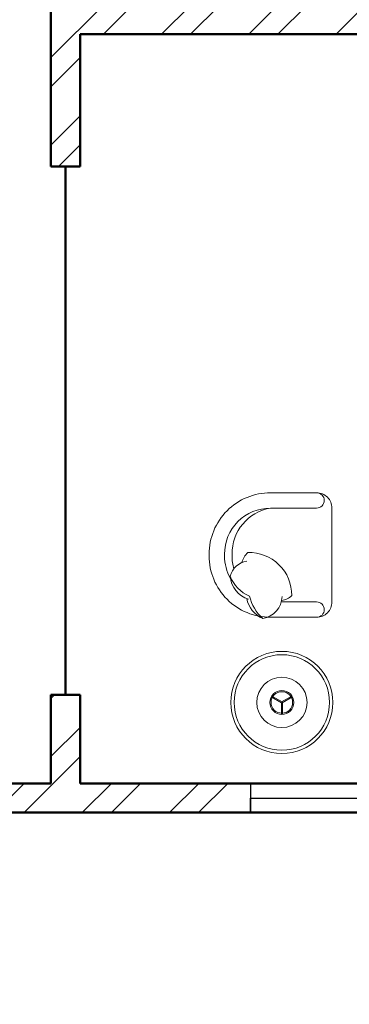
# Model space of a CAD drawing. Units: inches. Extents: x 1901 to 2863, y 888 to 2433.
# Tile 67 of 91: x 2601 to 2651, y 1732 to 1884. Entities that reach past the tile are written whole.
import ezdxf

# ---------------------------------------------------------------- set-up
doc = ezdxf.new("R2010")
doc.units = ezdxf.units.IN
for name, color, linetype, lineweight in [('A-FURN', 8, 'Continuous', 18), ('A-GLAZ', 3, 'Continuous', 25), ('A-WALL', 7, 'Continuous', 50), ('A-WALL-PATT', 8, 'Continuous', 13)]:
    doc.layers.add(name, color=color, linetype=linetype, lineweight=lineweight)

# ---------------------------------------------------------------- blocks, each defined once
blk = doc.blocks.new('WIN-60')
for p, q in [((0, 4.5), (0, 0)), ((60, 2.25), (60, 4.5)), ((60, 4.5), (60, 0)), ((0, 0), (0, 2.25)), ((0, 2.25), (60, 2.25))]:
    blk.add_line(p, q)

msp = doc.modelspace()

# ---------------------------------------------------------------- hatches: boundary and pattern name
at = {"layer": 'A-WALL-PATT'}
h = msp.add_hatch(dxfattribs=at)
h.set_pattern_fill('ANSI32', color=256)
h.paths.add_polyline_path([(2192.5, 2274.13), (2141.26, 2274.13), (2141.26, 2269.63), (2192.5, 2269.63)])
h.paths.add_polyline_path([(2259.93, 2274.13), (2216.5, 2274.13), (2216.5, 2269.63), (2255.43, 2269.63), (2255.43, 2214.63), (2250.81, 2214.63), (2250.81, 2210.13), (2259.93, 2210.13), (2259.93, 2215.13), (2271.76, 2215.13), (2271.76, 2217.38), (2271.76, 2219.63), (2259.93, 2219.63)])
h.paths.add_polyline_path([(2171.43, 2269.63), (2166.93, 2269.63), (2166.93, 2219.63), (2121.24, 2219.63), (2121.24, 2215.13), (2166.93, 2215.13), (2166.93, 2083.13), (2161.81, 2083.13), (2161.81, 2078.63), (2171.43, 2078.63), (2177, 2078.63), (2177, 2080.88), (2177, 2083.13), (2171.43, 2083.13), (2171.43, 2210.13), (2230.91, 2210.13), (2230.91, 2212.38), (2230.91, 2214.63), (2171.43, 2214.63)])
h.paths.add_polyline_path([(2117.26, 2274.13), (2089.43, 2274.13), (2089.43, 2219.63), (2081.14, 2219.63), (2081.14, 2215.13), (2089.43, 2215.13), (2098, 2215.13), (2098, 2217.38), (2098, 2219.63), (2093.93, 2219.63), (2093.93, 2269.63), (2117.26, 2269.63), (2117.26, 2271.88)])
h.paths.add_polyline_path([(2343.43, 2219.63), (2329.29, 2219.63), (2329.29, 2215.13), (2338.93, 2215.13), (2338.93, 2184.74), (2343.43, 2184.74)])
h.paths.add_polyline_path([(2338.93, 2083.13), (2329.29, 2083.13), (2208.97, 2083.13), (2208.97, 2078.63), (2338.93, 2078.63)])
h.paths.add_polyline_path([(2343.43, 2136.74), (2338.93, 2136.74), (2338.93, 1872.63), (2343.43, 1872.63)])
h.paths.add_polyline_path([(2343.43, 1863.63), (2397.68, 1863.63), (2397.68, 1821.63), (2384.14, 1821.63), (2384.14, 1812.63), (2418.33, 1812.63), (2418.33, 1817.13), (2418.33, 1821.63), (2406.68, 1821.63), (2406.68, 1863.63), (2459.5, 1863.63), (2459.5, 1821.63), (2447.14, 1821.63), (2447.14, 1812.63), (2459.5, 1812.63), (2468.5, 1812.63), (2468.5, 1872.63), (2394.43, 1872.63), (2334.43, 1872.63), (2334.43, 1812.63), (2343.43, 1812.63), (2353.25, 1812.63), (2353.25, 1821.63), (2343.43, 1821.63)])
h.paths.add_polyline_path([(2510.01, 1872.63), (2468.5, 1872.63), (2468.5, 1868.13), (2510.01, 1868.13)])
h.paths.add_polyline_path([(2514.01, 1817.13), (2468.5, 1817.13), (2468.5, 1812.63), (2482.11, 1812.63), (2482.11, 1800.61), (2486.61, 1800.61), (2486.61, 1812.63), (2514.01, 1812.63)])
h.paths.add_polyline_path([(2299.25, 1814.88), (2299.25, 1817.13), (2295.93, 1817.13), (2295.93, 1854.17), (2293.68, 1854.17), (2291.43, 1854.17), (2291.43, 1817.13), (2266.11, 1817.13), (2266.11, 1812.63), (2299.25, 1812.63)])
h.paths.add_polyline_path([(2218.11, 1817.13), (2206.46, 1817.13), (2171.43, 1817.13), (2171.43, 1949.13), (2190.1, 1949.13), (2190.1, 1953.63), (2163.47, 1953.63), (2163.47, 1949.13), (2166.93, 1949.13), (2166.93, 1817.13), (2114.3, 1817.13), (2114.3, 1812.63), (2218.11, 1812.63)])
h.paths.add_polyline_path([(2029.43, 1970.92), (2024.93, 1970.92), (2024.93, 1912.72), (2029.43, 1912.72)])
h.paths.add_polyline_path([(2132.3, 1953.63), (2113.93, 1953.63), (2113.93, 1975.89), (2111.68, 1975.89), (2109.43, 1975.89), (2109.43, 1953.63), (2029.43, 1953.63), (2029.43, 1949.13), (2132.3, 1949.13)])
h.paths.add_polyline_path([(2029.43, 1853.61), (2029.31, 1853.61), (2029.31, 1853.61), (2029.43, 1853.61), (2029.43, 1864.72), (2024.93, 1864.72), (2024.93, 1812.63), (2066.3, 1812.63), (2066.3, 1814.88), (2066.3, 1817.13), (2029.43, 1817.13)])
h.paths.add_polyline_path([(2122.93, 2010.09), (2120.68, 2010.09), (2118.43, 2010.09), (2118.43, 2006.13), (2029.43, 2006.13), (2029.43, 2001.63), (2109.43, 2001.63), (2109.43, 1998.04), (2113.93, 1998.04), (2113.93, 2001.63), (2122.93, 2001.63)])
h.paths.add_polyline_path([(2029.43, 2031.38), (2024.93, 2031.38), (2024.93, 1994.92), (2027.18, 1994.92), (2029.43, 1994.92)])
h.paths.add_polyline_path([(2029.43, 2136.74), (2024.93, 2136.74), (2024.93, 2067.38), (2027.18, 2067.38), (2029.43, 2067.38)])
h.paths.add_polyline_path([(2125.62, 2083.13), (2029.43, 2083.13), (2029.43, 2078.63), (2118.43, 2078.63), (2118.43, 2030.71), (2122.93, 2030.71), (2122.93, 2078.63), (2125.62, 2078.63)])
h.paths.add_polyline_path([(2029.43, 2215.13), (2040.47, 2215.13), (2040.47, 2217.38), (2040.47, 2219.63), (2024.93, 2219.63), (2024.93, 2184.74), (2029.43, 2184.74), (2029.43, 2187.78)])
h.paths.add_polyline_path([(2686.43, 2274.13), (2659.28, 2274.13), (2659.28, 2269.63), (2681.93, 2269.63), (2681.93, 2219.63), (2676.82, 2219.63), (2676.82, 2215.13), (2681.93, 2215.13), (2697.01, 2215.13), (2697.01, 2217.38), (2697.01, 2219.63), (2686.43, 2219.63)])
h.paths.add_polyline_path([(2609.93, 2269.63), (2635.28, 2269.63), (2635.28, 2274.13), (2571.43, 2274.13), (2571.43, 2269.63), (2605.43, 2269.63), (2605.43, 2214.63), (2549.1, 2214.63), (2549.1, 2210.13), (2605.43, 2210.13), (2605.43, 2083.13), (2601.01, 2083.13), (2601.01, 2080.88), (2601.01, 2078.63), (2609.93, 2078.63), (2616.16, 2078.63), (2616.16, 2080.88), (2616.16, 2083.13), (2609.93, 2083.13), (2609.93, 2215.13), (2651.46, 2215.13), (2651.46, 2217.38), (2651.46, 2219.63), (2609.93, 2219.63)])
h.paths.add_polyline_path([(2521.43, 2269.63), (2547.43, 2269.63), (2547.43, 2271.88), (2547.43, 2274.13), (2516.93, 2274.13), (2516.93, 2219.63), (2506.41, 2219.63), (2506.41, 2215.13), (2516.93, 2215.13), (2516.93, 2210.13), (2525.4, 2210.13), (2525.4, 2212.38), (2525.4, 2214.63), (2521.43, 2214.63)])
h.paths.add_polyline_path([(2456.01, 2219.63), (2439.43, 2219.63), (2439.43, 2187.89), (2443.93, 2187.89), (2443.93, 2215.13), (2456.01, 2215.13)])
h.paths.add_polyline_path([(2752.93, 2219.63), (2739.48, 2219.63), (2739.48, 2215.13), (2748.43, 2215.13), (2748.43, 2187.89), (2752.93, 2187.89)])
h.paths.add_polyline_path([(2752.93, 2139.89), (2748.43, 2139.89), (2748.43, 2083.13), (2648.42, 2083.13), (2648.42, 2078.63), (2654.93, 2078.63), (2654.93, 2039.44), (2659.43, 2039.44), (2659.43, 2078.63), (2748.43, 2078.63), (2748.43, 2063.43), (2752.93, 2063.43)])
h.paths.add_polyline_path([(2752.93, 2010.63), (2659.43, 2010.63), (2659.43, 2015.65), (2654.93, 2015.65), (2654.93, 2010.63), (2605.43, 2010.63), (2605.43, 1920.97), (2609.93, 1920.97), (2609.93, 2006.13), (2748.43, 2006.13), (2748.43, 1982.47), (2752.93, 1982.47)])
h.paths.add_polyline_path([(2752.93, 2027.43), (2748.43, 2027.43), (2748.43, 2010.63), (2752.93, 2010.63)])
h.paths.add_polyline_path([(2748.43, 1886.13), (2609.93, 1886.13), (2609.93, 1889.72), (2605.43, 1889.72), (2605.43, 1861.26), (2609.93, 1861.26), (2609.93, 1881.63), (2748.43, 1881.63)])
h.paths.add_polyline_path([(2456.86, 2228.83), (2498.4, 2228.83), (2498.4, 2247.49), (2456.86, 2247.49)], flags=9)
h.paths.add_polyline_path([(2038.6, 2237.42), (2080.17, 2237.42), (2080.17, 2256.08), (2038.6, 2256.08)], flags=9)
h.paths.add_polyline_path([(2292.01, 1062.39), (2539.93, 1062.39), (2539.93, 1099.49), (2292.01, 1099.49)], flags=9)
h.paths.add_polyline_path([(2424.91, 1832.25), (2448.51, 1832.25), (2448.51, 1846.68), (2424.91, 1846.68)], flags=25)
h.paths.add_polyline_path([(2359.08, 1832.25), (2382.68, 1832.25), (2382.68, 1846.68), (2359.08, 1846.68)], flags=25)
h.paths.add_polyline_path([(2352.9, 1684.8), (2367.54, 1684.8), (2367.54, 1697.17), (2352.9, 1697.17)], flags=9)
h.paths.add_polyline_path([(2079.29, 1755.83), (2169.02, 1755.83), (2169.02, 1774.37), (2079.29, 1774.37)], flags=9)
h.paths.add_polyline_path([(2404.09, 1373.86), (2404.09, 1463.59), (2385.54, 1463.59), (2385.54, 1373.86)], flags=9)
h.paths.add_polyline_path([(2268.09, 2236.37), (2309.64, 2236.37), (2309.64, 2255.03), (2268.09, 2255.03)], flags=9)
h.paths.add_polyline_path([(2575.96, 1700.95), (2665.7, 1700.95), (2665.7, 1719.5), (2575.96, 1719.5)], flags=9)
h.paths.add_polyline_path([(2302.96, 1878.47), (2329.52, 1878.47), (2329.52, 1888.78), (2302.96, 1888.78)], flags=9)
h.paths.add_polyline_path([(2097.42, 2240.58), (2126.57, 2240.58), (2126.57, 2259.23), (2097.42, 2259.23)], flags=9)
h.paths.add_polyline_path([(2208.72, 2246.12), (2237.88, 2246.12), (2237.88, 2264.78), (2208.72, 2264.78)], flags=9)
h.paths.add_polyline_path([(2038.15, 1925.96), (2076.99, 1925.96), (2076.99, 1944.62), (2038.15, 1944.62)], flags=9)
h.paths.add_polyline_path([(2239.14, 1926.67), (2288.46, 1926.67), (2288.46, 1945.33), (2239.14, 1945.33)], flags=9)
h.paths.add_polyline_path([(2175.43, 2007.33), (2212.36, 2007.33), (2212.36, 2025.99), (2175.43, 2025.99)], flags=9)
h.paths.add_polyline_path([(2225.03, 2091.79), (2263.87, 2091.79), (2263.87, 2110.45), (2225.03, 2110.45)], flags=9)
h.paths.add_polyline_path([(2035.4, 2098.48), (2074.24, 2098.48), (2074.24, 2117.14), (2035.4, 2117.14)], flags=9)
h.paths.add_polyline_path([(2050.1, 2029.21), (2083.26, 2029.21), (2083.26, 2047.87), (2050.1, 2047.87)], flags=9)
h.paths.add_polyline_path([(2069.68, 1956.72), (2098.83, 1956.72), (2098.83, 1975.38), (2069.68, 1975.38)], flags=25)
h.paths.add_polyline_path([(2328.62, 1753.34), (2361.66, 1753.34), (2361.66, 1771.99), (2328.62, 1771.99)], flags=9)
h.paths.add_polyline_path([(2395.16, 2060.89), (2395.16, 2140.65), (2378.68, 2140.65), (2378.68, 2060.89)], flags=9)
h.paths.add_polyline_path([(2463.73, 2059.02), (2492.89, 2059.02), (2492.89, 2077.68), (2463.73, 2077.68)], flags=9)
h.paths.add_polyline_path([(2458.03, 2181.54), (2496.87, 2181.54), (2496.87, 2200.19), (2458.03, 2200.19)], flags=9)
h.paths.add_polyline_path([(2527.58, 2243.07), (2556.73, 2243.07), (2556.73, 2261.73), (2527.58, 2261.73)], flags=9)
h.paths.add_polyline_path([(2694.46, 2232.77), (2736.03, 2232.77), (2736.03, 2251.42), (2694.46, 2251.42)], flags=9)
h.paths.add_polyline_path([(2637.82, 2249.22), (2666.98, 2249.22), (2666.98, 2267.88), (2637.82, 2267.88)], flags=9)
h.paths.add_polyline_path([(2623.69, 2183.54), (2662.53, 2183.54), (2662.53, 2202.2), (2623.69, 2202.2)], flags=9)
h.paths.add_polyline_path([(2691.97, 2021.5), (2725.12, 2021.5), (2725.12, 2040.16), (2691.97, 2040.16)], flags=9)
h.paths.add_polyline_path([(2621.04, 1975.91), (2662.34, 1975.91), (2662.34, 1994.57), (2621.04, 1994.57)], flags=25)
h.paths.add_polyline_path([(2479.03, 1927.62), (2519.84, 1927.62), (2519.84, 1946.28), (2479.03, 1946.28)], flags=9)
h.paths.add_polyline_path([(2670.94, 1849.08), (2716.01, 1849.08), (2716.01, 1867.73), (2670.94, 1867.73)], flags=9)
h.paths.add_polyline_path([(2523.61, 1782.96), (2550.17, 1782.96), (2550.17, 1793.26), (2523.61, 1793.26)], flags=9)
h.paths.add_polyline_path([(2450.84, 1207.33), (2492.39, 1207.33), (2492.39, 1225.99), (2450.84, 1225.99)], flags=9)
h.paths.add_polyline_path([(2527.75, 1203.84), (2556.91, 1203.84), (2556.91, 1222.5), (2527.75, 1222.5)], flags=9)
h.paths.add_polyline_path([(2639.11, 1207.2), (2668.27, 1207.2), (2668.27, 1225.86), (2639.11, 1225.86)], flags=9)
h.paths.add_polyline_path([(2692.59, 1218.97), (2734.17, 1218.97), (2734.17, 1237.62), (2692.59, 1237.62)], flags=9)
h.paths.add_polyline_path([(2669.27, 1366.33), (2708.11, 1366.33), (2708.11, 1384.99), (2669.27, 1384.99)], flags=9)
h.paths.add_polyline_path([(2463.31, 1358.03), (2502.15, 1358.03), (2502.15, 1376.69), (2463.31, 1376.69)], flags=9)
h.paths.add_polyline_path([(2494.72, 1449.96), (2531.65, 1449.96), (2531.65, 1468.62), (2494.72, 1468.62)], flags=9)
h.paths.add_polyline_path([(2675.57, 1422.16), (2708.72, 1422.16), (2708.72, 1440.81), (2675.57, 1440.81)], flags=9)
h.paths.add_polyline_path([(2685.63, 1493.89), (2714.79, 1493.89), (2714.79, 1512.55), (2685.63, 1512.55)], flags=9)
h.paths.add_polyline_path([(2686.8, 1529.91), (2725.65, 1529.91), (2725.65, 1548.57), (2686.8, 1548.57)], flags=9)
h.paths.add_polyline_path([(2503.65, 1537.99), (2552.97, 1537.99), (2552.97, 1556.65), (2503.65, 1556.65)], flags=9)
h.paths.add_polyline_path([(2291.71, 1643.5), (2318.28, 1643.5), (2318.28, 1653.81), (2291.71, 1653.81)], flags=9)
h.paths.add_polyline_path([(2450.63, 1610.52), (2477.19, 1610.52), (2477.19, 1620.82), (2450.63, 1620.82)], flags=9)
h.paths.add_polyline_path([(2359.99, 1551.81), (2422.25, 1551.81), (2422.25, 1562.12), (2359.99, 1562.12)], flags=9)
h.paths.add_polyline_path([(2280.11, 1249.01), (2321.65, 1249.01), (2321.65, 1267.66), (2280.11, 1267.66)], flags=9)
h.paths.add_polyline_path([(2164.06, 1274.23), (2193.22, 1274.23), (2193.22, 1292.89), (2164.06, 1292.89)], flags=9)
h.paths.add_polyline_path([(2118.21, 1277.69), (2151.25, 1277.69), (2151.25, 1296.35), (2118.21, 1296.35)], flags=9)
h.paths.add_polyline_path([(2031.95, 1268.53), (2073.52, 1268.53), (2073.52, 1287.19), (2031.95, 1287.19)], flags=9)
h.paths.add_polyline_path([(2050.2, 1409.08), (2089.04, 1409.08), (2089.04, 1427.74), (2050.2, 1427.74)], flags=9)
h.paths.add_polyline_path([(2243.74, 1421.03), (2282.58, 1421.03), (2282.58, 1439.69), (2243.74, 1439.69)], flags=9)
h.paths.add_polyline_path([(2190.75, 1509.77), (2231.56, 1509.77), (2231.56, 1528.43), (2190.75, 1528.43)], flags=9)
h.paths.add_polyline_path([(2058.39, 1475.42), (2091.55, 1475.42), (2091.55, 1494.07), (2058.39, 1494.07)], flags=9)
h.paths.add_polyline_path([(2062.45, 1553.09), (2091.6, 1553.09), (2091.6, 1571.75), (2062.45, 1571.75)], flags=9)
h.paths.add_polyline_path([(2219.52, 1590.37), (2266.15, 1590.37), (2266.15, 1609.02), (2219.52, 1609.02)], flags=9)
h.paths.add_polyline_path([(2041.07, 1584.19), (2079.91, 1584.19), (2079.91, 1602.85), (2041.07, 1602.85)], flags=9)
h = msp.add_hatch(dxfattribs=at)
h.set_pattern_fill('ANSI32', color=256)
h.paths.add_polyline_path([(2443.93, 2139.89), (2439.43, 2139.89), (2439.43, 2069.35), (2441.68, 2069.35), (2443.93, 2069.35), (2443.93, 2078.63), (2521.93, 2078.63), (2521.93, 2075.07), (2524.18, 2075.07), (2526.43, 2075.07), (2526.43, 2078.63), (2571.75, 2078.63), (2571.75, 2080.88), (2571.75, 2083.13), (2443.93, 2083.13)])
h.paths.add_polyline_path([(2526.43, 2054.63), (2524.18, 2054.63), (2521.93, 2054.63), (2521.93, 2030.63), (2443.93, 2030.63), (2443.93, 2045.35), (2439.43, 2045.35), (2439.43, 1983.87), (2443.93, 1983.87), (2443.93, 2026.13), (2521.93, 2026.13), (2526.43, 2026.13)])
h.paths.add_polyline_path([(2443.93, 1923.87), (2439.43, 1923.87), (2439.43, 1872.63), (2443.93, 1872.63)])
h.paths.add_polyline_path([(2636.23, 1766.13), (2609.93, 1766.13), (2609.93, 1779.79), (2605.43, 1779.79), (2605.43, 1766.13), (2486.61, 1766.13), (2486.61, 1770.67), (2482.11, 1770.67), (2482.11, 1766.13), (2482.11, 1761.63), (2636.23, 1761.63), (2636.23, 1763.88)])
h.paths.add_polyline_path([(2519.54, 1663.38), (2519.54, 1665.63), (2494.93, 1665.63), (2481.83, 1665.63), (2481.83, 1663.38), (2481.83, 1661.13), (2490.43, 1661.13), (2490.43, 1640.16), (2494.93, 1640.16), (2494.93, 1661.13), (2519.54, 1661.13)])
h.paths.add_polyline_path([(2443.93, 1712.13), (2443.93, 1716.63), (2414.46, 1716.63), (2414.46, 1712.13), (2439.43, 1712.13), (2439.43, 1545.51), (2443.93, 1545.51), (2443.93, 1661.13), (2448.47, 1661.13), (2448.47, 1665.63), (2443.93, 1665.63)])
h.paths.add_polyline_path([(2343.43, 1712.13), (2365.52, 1712.13), (2365.52, 1714.38), (2365.52, 1716.63), (2333.87, 1716.63), (2333.87, 1714.38), (2333.87, 1712.13), (2338.93, 1712.13), (2338.93, 1575.63), (2338.93, 1545.51), (2343.43, 1545.51), (2343.43, 1547.51), (2343.43, 1580.13)])
h.paths.add_polyline_path([(2752.93, 1665.63), (2579.54, 1665.63), (2579.54, 1661.13), (2615.93, 1661.13), (2615.93, 1529.13), (2598.93, 1529.13), (2598.93, 1524.63), (2623.13, 1524.63), (2623.13, 1526.88), (2623.13, 1529.13), (2620.43, 1529.13), (2620.43, 1661.13), (2748.43, 1661.13), (2748.43, 1633.5), (2752.93, 1633.5)])
h.paths.add_polyline_path([(2752.93, 1419.93), (2748.43, 1419.93), (2748.43, 1400.13), (2659.43, 1400.13), (2659.43, 1444.33), (2657.18, 1444.33), (2654.93, 1444.33), (2654.93, 1400.13), (2643.65, 1400.13), (2643.65, 1395.63), (2748.43, 1395.63), (2748.43, 1364.04), (2752.93, 1364.04)])
h.paths.add_polyline_path([(2752.93, 1492.88), (2748.43, 1492.88), (2748.43, 1476.63), (2667.43, 1476.63), (2667.43, 1479.71), (2665.18, 1479.71), (2662.93, 1479.71), (2662.93, 1476.63), (2654.93, 1476.63), (2654.93, 1469.54), (2659.43, 1469.54), (2659.43, 1472.13), (2748.43, 1472.13), (2748.43, 1455.93), (2752.93, 1455.93)])
h.paths.add_polyline_path([(2752.93, 1304.04), (2748.43, 1304.04), (2748.43, 1263.63), (2738.66, 1263.63), (2738.66, 1259.13), (2752.93, 1259.13)])
h.paths.add_polyline_path([(2685.93, 1259.13), (2695.49, 1259.13), (2695.49, 1261.38), (2695.49, 1263.63), (2677.84, 1263.63), (2677.84, 1261.38), (2677.84, 1259.13), (2681.43, 1259.13), (2681.43, 1203.63), (2653.28, 1203.63), (2653.28, 1199.13), (2685.93, 1199.13), (2685.93, 1203.63)])
h.paths.add_polyline_path([(2609.43, 1395.63), (2611.85, 1395.63), (2611.85, 1400.13), (2598.89, 1400.13), (2598.89, 1397.88), (2598.89, 1395.63), (2604.93, 1395.63), (2604.93, 1268.13), (2554.73, 1268.13), (2554.73, 1265.88), (2554.73, 1263.63), (2604.93, 1263.63), (2604.93, 1203.63), (2571.31, 1203.63), (2571.31, 1199.13), (2604.93, 1199.13), (2629.28, 1199.13), (2629.28, 1201.38), (2629.28, 1203.63), (2609.43, 1203.63), (2609.43, 1258.63), (2609.43, 1259.13), (2654.8, 1259.13), (2654.8, 1263.63), (2609.43, 1263.63)])
h.paths.add_polyline_path([(2443.93, 1304.04), (2439.43, 1304.04), (2439.43, 1259.13), (2443.93, 1259.13), (2456.16, 1259.13), (2456.16, 1261.38), (2456.16, 1263.63), (2443.93, 1263.63)])
h.paths.add_polyline_path([(2525.43, 1263.63), (2531.78, 1263.63), (2531.78, 1268.13), (2520.93, 1268.13), (2520.93, 1263.63), (2511.41, 1263.63), (2511.41, 1259.13), (2520.93, 1259.13), (2520.93, 1199.13), (2547.31, 1199.13), (2547.31, 1201.38), (2547.31, 1203.63), (2525.43, 1203.63)])
h.paths.add_polyline_path([(2443.93, 1434.84), (2439.43, 1434.84), (2439.43, 1364.04), (2441.68, 1364.04), (2443.93, 1364.04)])
h.paths.add_polyline_path([(2567.13, 1400.13), (2443.93, 1400.13), (2443.93, 1395.63), (2567.13, 1395.63)])
h.paths.add_polyline_path([(2443.93, 1545.51), (2439.43, 1545.51), (2439.43, 1494.84), (2443.93, 1494.84)])
h.paths.add_polyline_path([(2494.93, 1553.35), (2492.68, 1553.35), (2490.43, 1553.35), (2490.43, 1524.63), (2494.93, 1524.63), (2525.94, 1524.63), (2525.94, 1526.88), (2525.94, 1529.13), (2494.93, 1529.13)])
h.paths.add_polyline_path([(2752.93, 1573.5), (2748.43, 1573.5), (2748.43, 1529.13), (2657.76, 1529.13), (2657.76, 1524.63), (2662.93, 1524.63), (2662.93, 1498.63), (2667.43, 1498.63), (2667.43, 1524.63), (2748.43, 1524.63), (2748.43, 1516.88), (2752.93, 1516.88)])
h.paths.add_polyline_path([(2038.6, 2237.42), (2080.17, 2237.42), (2080.17, 2256.08), (2038.6, 2256.08)], flags=9)
h.paths.add_polyline_path([(2292.01, 1062.39), (2539.93, 1062.39), (2539.93, 1099.49), (2292.01, 1099.49)], flags=9)
h.paths.add_polyline_path([(2424.91, 1832.25), (2448.51, 1832.25), (2448.51, 1846.68), (2424.91, 1846.68)], flags=9)
h.paths.add_polyline_path([(2359.08, 1832.25), (2382.68, 1832.25), (2382.68, 1846.68), (2359.08, 1846.68)], flags=9)
h.paths.add_polyline_path([(2352.9, 1684.8), (2367.54, 1684.8), (2367.54, 1697.17), (2352.9, 1697.17)], flags=9)
h.paths.add_polyline_path([(2079.29, 1755.83), (2169.02, 1755.83), (2169.02, 1774.37), (2079.29, 1774.37)], flags=9)
h.paths.add_polyline_path([(2404.09, 1373.86), (2404.09, 1463.59), (2385.54, 1463.59), (2385.54, 1373.86)], flags=9)
h.paths.add_polyline_path([(2268.09, 2236.37), (2309.64, 2236.37), (2309.64, 2255.03), (2268.09, 2255.03)], flags=9)
h.paths.add_polyline_path([(2575.96, 1700.95), (2665.7, 1700.95), (2665.7, 1719.5), (2575.96, 1719.5)], flags=9)
h.paths.add_polyline_path([(2302.96, 1878.47), (2329.52, 1878.47), (2329.52, 1888.78), (2302.96, 1888.78)], flags=9)
h.paths.add_polyline_path([(2097.42, 2240.58), (2126.57, 2240.58), (2126.57, 2259.23), (2097.42, 2259.23)], flags=9)
h.paths.add_polyline_path([(2208.72, 2246.12), (2237.88, 2246.12), (2237.88, 2264.78), (2208.72, 2264.78)], flags=9)
h.paths.add_polyline_path([(2038.15, 1925.96), (2076.99, 1925.96), (2076.99, 1944.62), (2038.15, 1944.62)], flags=9)
h.paths.add_polyline_path([(2239.14, 1926.67), (2288.46, 1926.67), (2288.46, 1945.33), (2239.14, 1945.33)], flags=9)
h.paths.add_polyline_path([(2175.43, 2007.33), (2212.36, 2007.33), (2212.36, 2025.99), (2175.43, 2025.99)], flags=9)
h.paths.add_polyline_path([(2225.03, 2091.79), (2263.87, 2091.79), (2263.87, 2110.45), (2225.03, 2110.45)], flags=9)
h.paths.add_polyline_path([(2035.4, 2098.48), (2074.24, 2098.48), (2074.24, 2117.14), (2035.4, 2117.14)], flags=9)
h.paths.add_polyline_path([(2050.1, 2029.21), (2083.26, 2029.21), (2083.26, 2047.87), (2050.1, 2047.87)], flags=9)
h.paths.add_polyline_path([(2069.68, 1956.72), (2098.83, 1956.72), (2098.83, 1975.38), (2069.68, 1975.38)], flags=9)
h.paths.add_polyline_path([(2328.62, 1753.34), (2361.66, 1753.34), (2361.66, 1771.99), (2328.62, 1771.99)], flags=9)
h.paths.add_polyline_path([(2395.16, 2060.89), (2395.16, 2140.65), (2378.68, 2140.65), (2378.68, 2060.89)], flags=9)
h.paths.add_polyline_path([(2463.73, 2059.02), (2492.89, 2059.02), (2492.89, 2077.68), (2463.73, 2077.68)], flags=9)
h.paths.add_polyline_path([(2458.03, 2181.54), (2496.87, 2181.54), (2496.87, 2200.19), (2458.03, 2200.19)], flags=9)
h.paths.add_polyline_path([(2456.86, 2228.83), (2498.4, 2228.83), (2498.4, 2247.49), (2456.86, 2247.49)], flags=9)
h.paths.add_polyline_path([(2527.58, 2243.07), (2556.73, 2243.07), (2556.73, 2261.73), (2527.58, 2261.73)], flags=9)
h.paths.add_polyline_path([(2694.46, 2232.77), (2736.03, 2232.77), (2736.03, 2251.42), (2694.46, 2251.42)], flags=9)
h.paths.add_polyline_path([(2637.82, 2249.22), (2666.98, 2249.22), (2666.98, 2267.88), (2637.82, 2267.88)], flags=9)
h.paths.add_polyline_path([(2623.69, 2183.54), (2662.53, 2183.54), (2662.53, 2202.2), (2623.69, 2202.2)], flags=9)
h.paths.add_polyline_path([(2691.97, 2021.5), (2725.12, 2021.5), (2725.12, 2040.16), (2691.97, 2040.16)], flags=9)
h.paths.add_polyline_path([(2621.04, 1975.91), (2662.34, 1975.91), (2662.34, 1994.57), (2621.04, 1994.57)], flags=9)
h.paths.add_polyline_path([(2479.03, 1927.62), (2519.84, 1927.62), (2519.84, 1946.28), (2479.03, 1946.28)], flags=9)
h.paths.add_polyline_path([(2670.94, 1849.08), (2716.01, 1849.08), (2716.01, 1867.73), (2670.94, 1867.73)], flags=9)
h.paths.add_polyline_path([(2523.61, 1782.96), (2550.17, 1782.96), (2550.17, 1793.26), (2523.61, 1793.26)], flags=9)
h.paths.add_polyline_path([(2450.84, 1207.33), (2492.39, 1207.33), (2492.39, 1225.99), (2450.84, 1225.99)], flags=9)
h.paths.add_polyline_path([(2527.75, 1203.84), (2556.91, 1203.84), (2556.91, 1222.5), (2527.75, 1222.5)], flags=9)
h.paths.add_polyline_path([(2639.11, 1207.2), (2668.27, 1207.2), (2668.27, 1225.86), (2639.11, 1225.86)], flags=9)
h.paths.add_polyline_path([(2692.59, 1218.97), (2734.17, 1218.97), (2734.17, 1237.62), (2692.59, 1237.62)], flags=9)
h.paths.add_polyline_path([(2669.27, 1366.33), (2708.11, 1366.33), (2708.11, 1384.99), (2669.27, 1384.99)], flags=25)
h.paths.add_polyline_path([(2463.31, 1358.03), (2502.15, 1358.03), (2502.15, 1376.69), (2463.31, 1376.69)], flags=9)
h.paths.add_polyline_path([(2494.72, 1449.96), (2531.65, 1449.96), (2531.65, 1468.62), (2494.72, 1468.62)], flags=9)
h.paths.add_polyline_path([(2675.57, 1422.16), (2708.72, 1422.16), (2708.72, 1440.81), (2675.57, 1440.81)], flags=25)
h.paths.add_polyline_path([(2685.63, 1493.89), (2714.79, 1493.89), (2714.79, 1512.55), (2685.63, 1512.55)], flags=9)
h.paths.add_polyline_path([(2686.8, 1529.91), (2725.65, 1529.91), (2725.65, 1548.57), (2686.8, 1548.57)], flags=25)
h.paths.add_polyline_path([(2503.65, 1537.99), (2552.97, 1537.99), (2552.97, 1556.65), (2503.65, 1556.65)], flags=9)
h.paths.add_polyline_path([(2291.71, 1643.5), (2318.28, 1643.5), (2318.28, 1653.81), (2291.71, 1653.81)], flags=9)
h.paths.add_polyline_path([(2450.63, 1610.52), (2477.19, 1610.52), (2477.19, 1620.82), (2450.63, 1620.82)], flags=9)
h.paths.add_polyline_path([(2359.99, 1551.81), (2422.25, 1551.81), (2422.25, 1562.12), (2359.99, 1562.12)], flags=9)
h.paths.add_polyline_path([(2280.11, 1249.01), (2321.65, 1249.01), (2321.65, 1267.66), (2280.11, 1267.66)], flags=9)
h.paths.add_polyline_path([(2164.06, 1274.23), (2193.22, 1274.23), (2193.22, 1292.89), (2164.06, 1292.89)], flags=9)
h.paths.add_polyline_path([(2118.21, 1277.69), (2151.25, 1277.69), (2151.25, 1296.35), (2118.21, 1296.35)], flags=9)
h.paths.add_polyline_path([(2031.95, 1268.53), (2073.52, 1268.53), (2073.52, 1287.19), (2031.95, 1287.19)], flags=9)
h.paths.add_polyline_path([(2050.2, 1409.08), (2089.04, 1409.08), (2089.04, 1427.74), (2050.2, 1427.74)], flags=9)
h.paths.add_polyline_path([(2243.74, 1421.03), (2282.58, 1421.03), (2282.58, 1439.69), (2243.74, 1439.69)], flags=9)
h.paths.add_polyline_path([(2190.75, 1509.77), (2231.56, 1509.77), (2231.56, 1528.43), (2190.75, 1528.43)], flags=9)
h.paths.add_polyline_path([(2058.39, 1475.42), (2091.55, 1475.42), (2091.55, 1494.07), (2058.39, 1494.07)], flags=9)
h.paths.add_polyline_path([(2062.45, 1553.09), (2091.6, 1553.09), (2091.6, 1571.75), (2062.45, 1571.75)], flags=9)
h.paths.add_polyline_path([(2219.52, 1590.37), (2266.15, 1590.37), (2266.15, 1609.02), (2219.52, 1609.02)], flags=9)
h.paths.add_polyline_path([(2041.07, 1584.19), (2079.91, 1584.19), (2079.91, 1602.85), (2041.07, 1602.85)], flags=9)

# ---------------------------------------------------------------- linework, layer by layer
at = {"layer": 'A-FURN', "ltscale": 0.03}
for p, q in [((2641.03, 1778.55), (2639.42, 1779.47)), ((2641.11, 1778.69), (2639.51, 1779.61)), ((2641.03, 1778.69), (2642.63, 1779.61)), ((2641.11, 1778.55), (2642.72, 1779.47)), ((2640.99, 1778.62), (2640.99, 1776.76)), ((2641.15, 1778.62), (2641.15, 1776.76))]:
    msp.add_line(p, q, dxfattribs=at)
msp.add_lwpolyline([(2648.79, 1801.35), (2648.79, 1808.58, 0.414214), (2646.43, 1810.95), (2639.32, 1810.95, 0.414214), (2629.84, 1801.47), (2629.84, 1801.35), (2629.84, 1801.23, 0.414214), (2639.32, 1791.75), (2646.43, 1791.75, 0.414214), (2648.79, 1794.12), (2648.79, 1801.35)], format="xyb", dxfattribs=at)
at = {"layer": 'A-FURN'}
for points in [[(2639.32, 1808.58), (2646.43, 1808.58, 0.414214), (2647.61, 1809.76), (2647.61, 1809.76, 0.414214), (2646.43, 1810.95)], [(2639.32, 1808.58, 0.414214), (2632.21, 1801.47), (2632.21, 1801.35)], [(2639.32, 1808.58, 0.372719), (2633.39, 1801.47), (2633.39, 1801.35)], [(2633.15, 1797.7, -0.130591), (2632.21, 1801.23), (2632.21, 1801.35)], [(2635.92, 1794.54, -0.306663), (2633.1, 1798.08, -0.30633), (2635.68, 1800.39, 0.872847)], [(2633.65, 1799.21, -0.072384), (2633.39, 1801.23), (2633.39, 1801.35)], [(2641.03, 1794.36, 0.165541), (2642.6, 1795.09, 0.425989), (2635.81, 1801.74, 0.121523), (2634.88, 1800.16, -7.115464)], [(2638.12, 1791.56, -0.14773), (2636.08, 1795.02, -0.213343), (2633.1, 1798.08, -0.178662)], [(2641.11, 1794.95, -0.356772), (2638.12, 1791.56, -0.249542), (2635.66, 1794.63, 9.61688)], [(2640.98, 1794.12), (2646.43, 1794.12, -0.414214), (2647.61, 1792.94), (2647.61, 1792.94, -0.414214), (2646.43, 1791.75)]]:
    msp.add_lwpolyline(points, format="xyb", dxfattribs=at)
at = {"layer": 'A-FURN', "ltscale": 0.03}
for radius in [7.88, 3.88, 1.85, 1.66]:
    msp.add_circle((2641.07, 1778.62), radius, dxfattribs=at)
at = {"layer": 'A-FURN'}
msp.add_circle((2641.07, 1778.62), 7.36, dxfattribs=at)
at = {"layer": 'A-WALL'}
for p, q in [((2605.43, 1889.72), (2605.43, 1861.26)), ((2609.93, 1881.63), (2748.43, 1881.63)), ((2609.93, 1881.63), (2609.93, 1861.26)), ((2609.93, 1881.63), (2609.93, 1861.26)), ((2605.43, 1864.84), (2605.43, 1864.84)), ((2605.43, 1861.26), (2609.93, 1861.26)), ((2607.68, 1861.26), (2607.68, 1779.79)), ((2605.43, 1766.13), (2605.43, 1779.79)), ((2605.43, 1779.79), (2609.93, 1779.79)), ((2609.93, 1779.79), (2609.93, 1766.13)), ((2605.43, 1766.13), (2486.61, 1766.13)), ((2748.43, 1766.13), (2609.93, 1766.13)), ((2482.11, 1761.63), (2752.93, 1761.63))]:
    msp.add_line(p, q, dxfattribs=at)

# ---------------------------------------------------------------- block references
at = {"layer": 'A-GLAZ'}
msp.add_blockref('WIN-60', (2636.23, 1761.63), dxfattribs=at)

doc.saveas('drawing.dxf')
